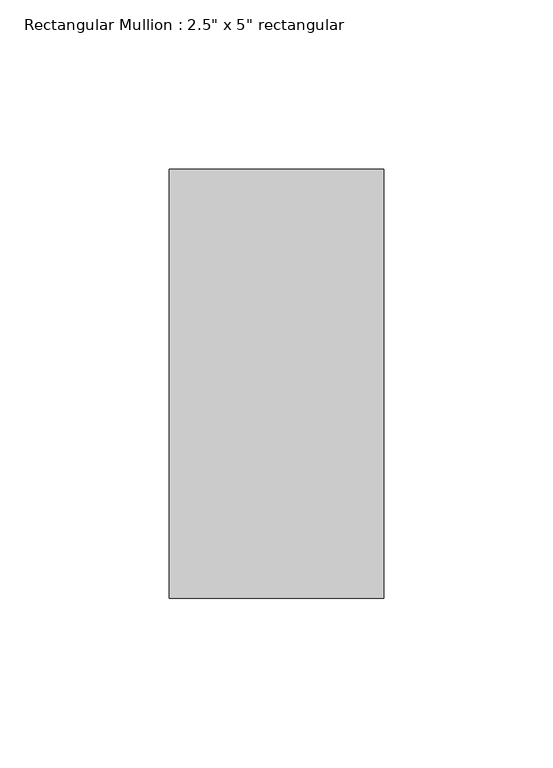
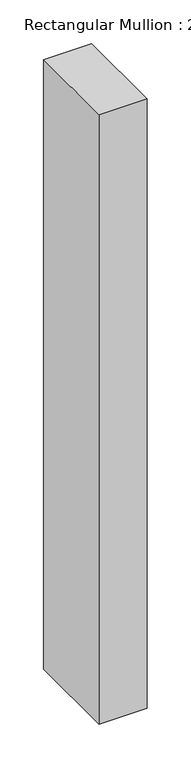
"""IFC4 building model written with IfcOpenShell, lengths in millimetres: member geometry."""

from ifc_helpers import new_model, si_unit, frame, origin, place, context, project, spatial, polyline, outline, extrude, source, transform, mapped, element, save


def member_7db1855a(model_context):
    return source(origin(), model_context, "Body", "SweptSolid", [
        extrude(outline(polyline([(31.75, 63.5), (31.75, -63.5), (-31.75, -63.5), (-31.75, 63.5), (31.75, 63.5)])), frame((0.0, 0.0, -850.9), z_axis=(0.0, 0.0, 1.0), x_axis=(1.0, 0.0, 0.0)), (0.0, 0.0, 1.0), 850.9),
    ])


if __name__ == "__main__":
    model = new_model("IFC4")
    model_context = context("Model", 3, world=origin())
    ifc_project = project(units=[si_unit("LENGTHUNIT", "METRE", prefix="MILLI")], contexts=[model_context])
    site = spatial("IfcSite", under=ifc_project)
    building = spatial("IfcBuilding", under=site)
    placement = place(None, origin())
    member_shape = member_7db1855a(model_context)
    element("IfcMember", 1, ObjectType="Rectangular Mullion : 2.5\" x 5\" rectangular", at=placement, inside=building, context=model_context, shape_type="MappedRepresentation", body=[
        mapped(member_shape, transform((0.0, 0.0, 0.0), x_axis=(1.0, 0.0, 0.0), y_axis=(0.0, 1.0, 0.0), z_axis=(0.0, 0.0, 1.0))),
    ])
    save(model, "model.ifc")

# Revit data of these elements
# Type "Rectangular Mullion : 2.5\" x 5\" rectangular"
#   built-in parameter 1007304 = 0.416667 (stored number, unit not read)
#   built-in parameter 1007301 = 0.104167 (stored number, unit not read)
#   built-in parameter 1007300 = 0.104167 (stored number, unit not read)
# Element 1 (IfcMember, "Rectangular Mullion : 2.5\" x 5\" rectangular")
#   Materials on its faces: "Aluminum"
# Materials
#   "Aluminum": class "Metal", colour RGB 247 247 247, transparency 0, Description = "Aluminum 6061", Cost = 0
